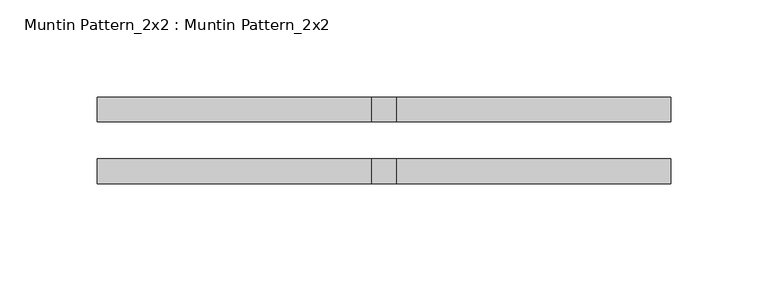
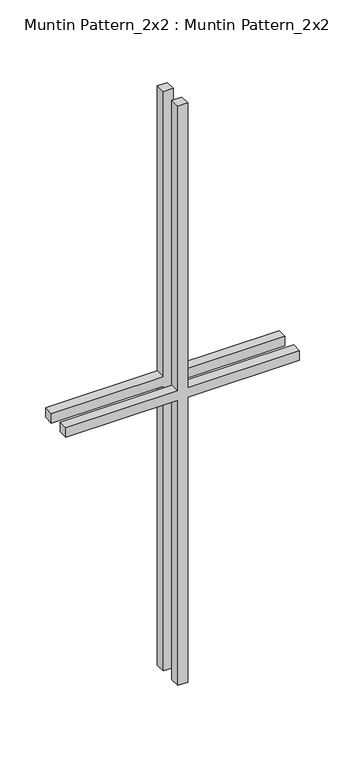
"""IFC4 building model written with IfcOpenShell, lengths in millimetres: proxy geometry, Muntin Pattern_2x2 : Muntin Pattern_2x2."""

from ifc_helpers import new_model, si_unit, frame, origin, place, context, project, spatial, polyline, outline, extrude, source, transform, mapped, element, save


def muntin_pattern_2x2_muntin_pattern_2x2_3e0ecaf2(model_context):
    return source(origin(), model_context, "Body", "SweptSolid", [
        extrude(outline(polyline([(393.7, -6.35), (393.7, -147.6375), (381.0, -147.6375), (381.0, -6.35), (0.0, -6.35), (0.0, 6.35), (381.0, 6.35), (381.0, 147.6375), (393.7, 147.6375), (393.7, 6.35), (774.7, 6.35), (774.7, -6.35), (393.7, -6.35)])), frame((0.0, -22.225, 0.0), z_axis=(0.0, 1.0, 0.0), x_axis=(0.0, 0.0, 1.0)), (0.0, 0.0, 1.0), 12.7),
        extrude(outline(polyline([(393.7, -6.35), (393.7, -147.6375), (381.0, -147.6375), (381.0, -6.35), (0.0, -6.35), (0.0, 6.35), (381.0, 6.35), (381.0, 147.6375), (393.7, 147.6375), (393.7, 6.35), (774.7, 6.35), (774.7, -6.35), (393.7, -6.35)])), frame((0.0, 9.525, 0.0), z_axis=(0.0, 1.0, 0.0), x_axis=(0.0, 0.0, 1.0)), (0.0, 0.0, 1.0), 12.7),
    ])


if __name__ == "__main__":
    model = new_model("IFC4")
    model_context = context("Model", 3, world=origin())
    ifc_project = project(units=[si_unit("LENGTHUNIT", "METRE", prefix="MILLI")], contexts=[model_context])
    site = spatial("IfcSite", under=ifc_project)
    building = spatial("IfcBuilding", under=site)
    placement = place(None, origin())
    muntin_pattern_2x2_muntin_pattern_2x2_shape = muntin_pattern_2x2_muntin_pattern_2x2_3e0ecaf2(model_context)
    element("IfcBuildingElementProxy", 1, Name="Muntin Pattern_2x2 : Muntin Pattern_2x2", ObjectType="Muntin Pattern_2x2 : Muntin Pattern_2x2", at=placement, inside=building, context=model_context, shape_type="MappedRepresentation", body=[
        mapped(muntin_pattern_2x2_muntin_pattern_2x2_shape, transform((0.0, 0.0, 0.0), x_axis=(1.0, 0.0, 0.0), y_axis=(0.0, 1.0, 0.0), z_axis=(0.0, 0.0, 1.0))),
    ])
    save(model, "model.ifc")

# Revit data of these elements
# Type "Muntin Pattern_2x2 : Muntin Pattern_2x2"
#   Width [instance default] = 4' - 0"
#   Thickness = 0' - 0 1/2"
#   Height [instance default] = 4' - 0"
#   Distance = 0' - 0 3/4"
#   Interior Material [instance default] = none
#   Exterior Material [instance default] = none
#   Default Elevation = 0
# Element 1 (IfcBuildingElementProxy, "Muntin Pattern_2x2 : Muntin Pattern_2x2")
#   Width = 0' - 11 5/8"
#   Height = 2' - 6 1/2"
#   Interior Material = Wood - Stained
#   Exterior Material = Clad - White
#   Materials on its faces: "Clad - White", "Wood - Stained"
# Materials
#   "Clad - White": class "Wood", colour RGB 242 242 238, transparency 0, Cost = 0
#   "Wood - Stained": class "Wood", colour RGB 224 178 126, transparency 0, Cost = 0
